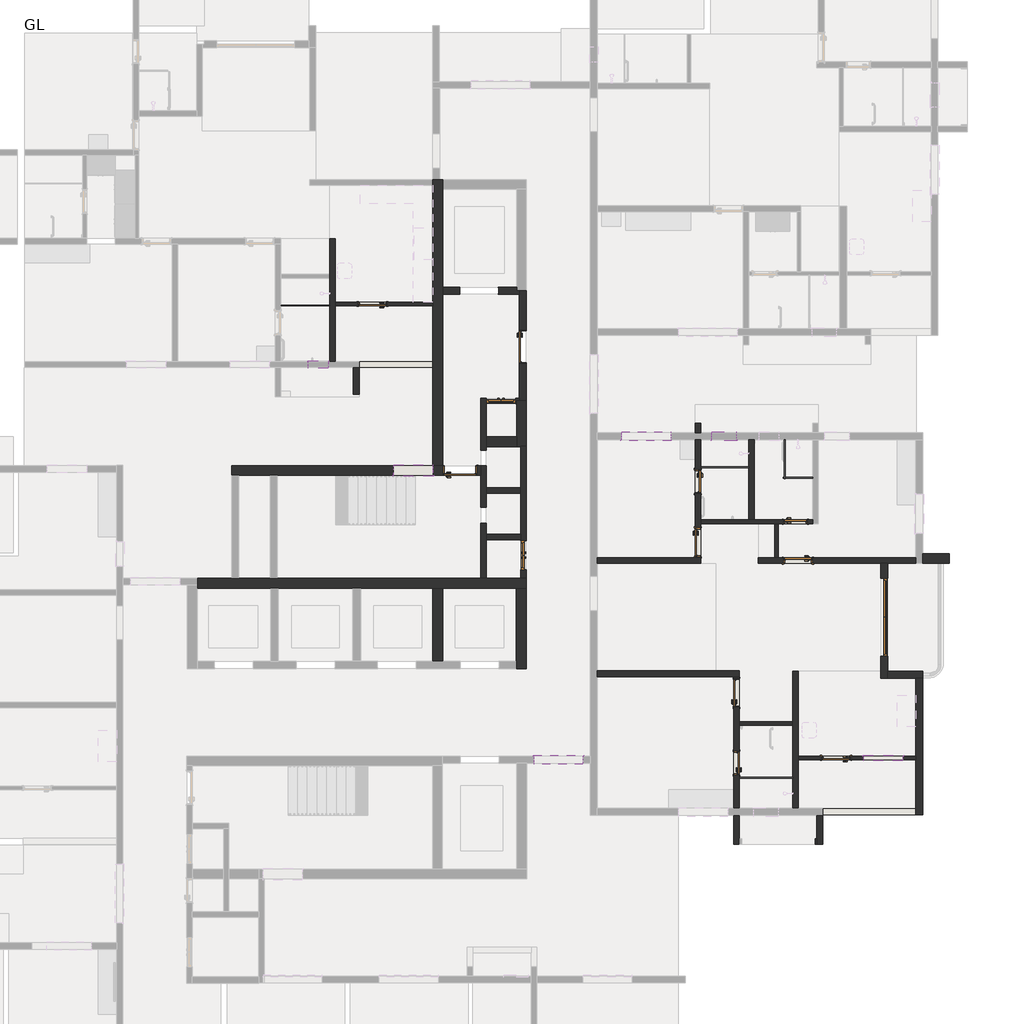
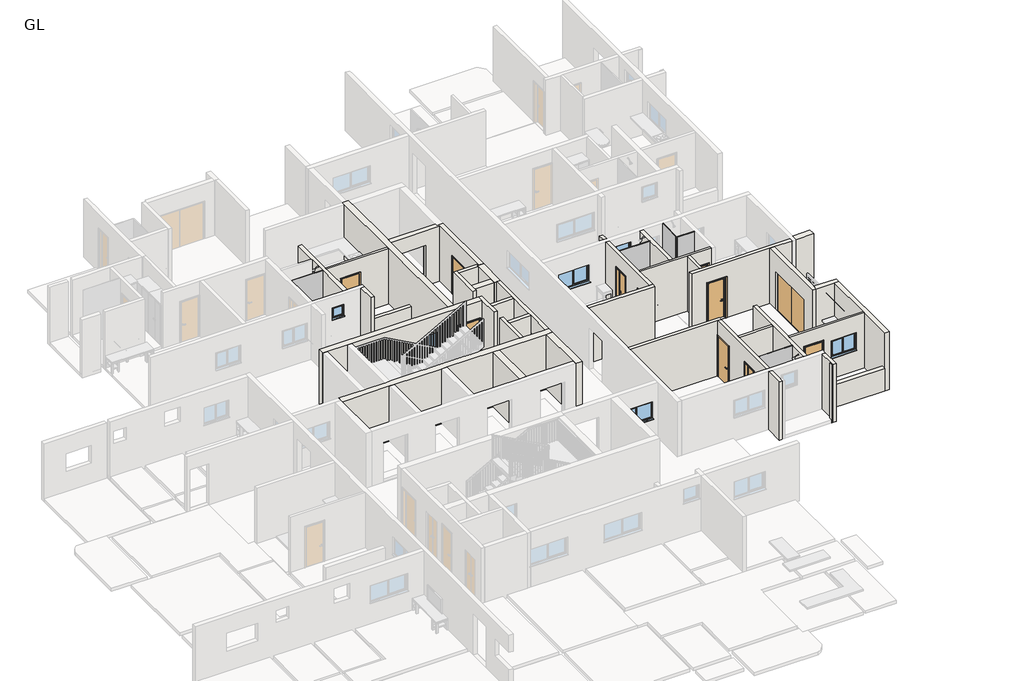
# One storey, part 5 of 14: 39 walls, 13 doors, 6 windows, 5 plates.
"""IFC4 building model written with IfcOpenShell, lengths in millimetres."""

from ifc_helpers import new_model, si_unit, frame, origin, origin_with_axes, place, context, project, spatial, polyline, outline, extrude, faceted_brep, transform, mapped, element, save
from components import doors_concept_extdbl_8_449e5563, doors_extdbl_flush_3_1e4ff7a8, doors_intsgl_2_5_door_21b53886, doors_intsgl_2_5_door_ce04bd24, doors_intsgl_2_5_door_fd097d29, doors_intsgl_3_door_8261d8fb, doors_intsgl_3_door_f61d7fb9, doors_intsgl_3_door_77e94e6e, doors_intsgl_3_5_f2e8c556, doors_intsgl_3_5_83ebdd9c, system_panel_glazed_f5bfe384, system_panel_glazed_a7f3818b, system_panel_glazed_4e5522aa, system_panel_glazed_8fd4c810, system_panel_glazed_557224e7, windows_dbl_plain_4_ad201dc9, windows_dbl_plain_4_4767a56f, windows_dbl_plain_5_907a13a5, windows_dbl_plain_5_93ba300c, windows_sgl_plain_2_43817c1b, windows_sgl_plain_2_5_21186da1

model = new_model("IFC4")

# Units and contexts
model_context = context("Model", 3, world=origin())
ifc_project = project(units=[si_unit("LENGTHUNIT", "METRE", prefix="MILLI")], contexts=[model_context])

# Site, building, storey
site = spatial("IfcSite", under=ifc_project)
building = spatial("IfcBuilding", under=site)
storey = spatial("IfcBuildingStorey", under=building, Name="GL", Elevation=0.0)

# Doors
placement = place(None, origin())
doors_concept_extdbl_8_shape = doors_concept_extdbl_8_449e5563(model_context)
element("IfcDoor", 1, ObjectType="Doors_Concept_ExtDbl : 8'", at=placement, inside=storey, context=model_context, shape_type="MappedRepresentation", body=[
    mapped(doors_concept_extdbl_8_shape, transform((18469.2769726, 77729.0878957, 0.0), x_axis=(0.0, -1.0, 0.0), y_axis=(1.0, 0.0, 0.0), z_axis=(0.0, 0.0, 1.0))),
])
doors_extdbl_flush_3_shape = doors_extdbl_flush_3_1e4ff7a8(model_context)
element("IfcDoor", 2, ObjectType="Doors_ExtDbl_Flush : 3'", at=placement, inside=storey, context=model_context, shape_type="MappedRepresentation", body=[
    mapped(doors_extdbl_flush_3_shape, transform((6505.8928654, 84487.5807724, 0.0), x_axis=(-1.0, 0.0, 0.0), y_axis=(0.0, -1.0, 0.0), z_axis=(0.0, 0.0, 1.0))),
])
element("IfcDoor", 3, ObjectType="Doors_ExtDbl_Flush : 3'", at=placement, inside=storey, context=model_context, shape_type="MappedRepresentation", body=[
    mapped(doors_extdbl_flush_3_shape, transform((7204.1388654, 79670.2853985, 0.0), x_axis=(0.0, 1.0, 0.0), y_axis=(-1.0, 0.0, 0.0), z_axis=(0.0, 0.0, 1.0))),
])
doors_intsgl_2_5_door_shape = doors_intsgl_2_5_door_21b53886(model_context)
element("IfcDoor", 4, ObjectType="Doors_IntSgl : 2.5' DOOR", at=placement, inside=storey, context=model_context, shape_type="MappedRepresentation", body=[
    mapped(doors_intsgl_2_5_door_shape, transform((15698.5624579, 80714.8578957, 149.9616), x_axis=(1.0, 0.0, 0.0), y_axis=(0.0, 1.0, 0.0), z_axis=(0.0, 0.0, 1.0))),
])
doors_intsgl_2_5_door_2_shape = doors_intsgl_2_5_door_ce04bd24(model_context)
element("IfcDoor", 5, ObjectType="Doors_IntSgl : 2.5' DOOR", at=placement, inside=storey, context=model_context, shape_type="MappedRepresentation", body=[
    mapped(doors_intsgl_2_5_door_2_shape, transform((12650.3084579, 81965.8078957, 149.9616), x_axis=(0.0, -1.0, 0.0), y_axis=(1.0, 0.0, 0.0), z_axis=(0.0, 0.0, 1.0))),
])
doors_intsgl_2_5_door_3_shape = doors_intsgl_2_5_door_fd097d29(model_context)
element("IfcDoor", 6, ObjectType="Doors_IntSgl : 2.5' DOOR", at=placement, inside=storey, context=model_context, shape_type="MappedRepresentation", body=[
    mapped(doors_intsgl_2_5_door_3_shape, transform((13856.9483556, 73179.9478957, 149.9616), x_axis=(0.0, 1.0, 0.0), y_axis=(-1.0, 0.0, 0.0), z_axis=(0.0, 0.0, 1.0))),
])
doors_intsgl_3_door_shape = doors_intsgl_3_door_8261d8fb(model_context)
element("IfcDoor", 7, ObjectType="Doors_IntSgl : 3' DOOR", at=placement, inside=storey, context=model_context, shape_type="MappedRepresentation", body=[
    mapped(doors_intsgl_3_door_shape, transform((12650.3084579, 80069.4438957, 149.9616), x_axis=(0.0, -1.0, 0.0), y_axis=(1.0, 0.0, 0.0), z_axis=(0.0, 0.0, 1.0))),
])
element("IfcDoor", 8, ObjectType="Doors_IntSgl : 3' DOOR", at=placement, inside=storey, context=model_context, shape_type="MappedRepresentation", body=[
    mapped(doors_intsgl_3_door_shape, transform((15774.7624579, 79499.9758957, 149.9616), x_axis=(-1.0, 0.0, 0.0), y_axis=(0.0, -1.0, 0.0), z_axis=(0.0, 0.0, 1.0))),
])
doors_intsgl_3_door_2_shape = doors_intsgl_3_door_f61d7fb9(model_context)
element("IfcDoor", 9, ObjectType="Doors_IntSgl : 3' DOOR", at=placement, inside=storey, context=model_context, shape_type="MappedRepresentation", body=[
    mapped(doors_intsgl_3_door_2_shape, transform((13856.9483556, 75373.5131416, 149.9616), x_axis=(0.0, 1.0, 0.0), y_axis=(-1.0, 0.0, 0.0), z_axis=(0.0, 0.0, 1.0))),
])
doors_intsgl_3_door_3_shape = doors_intsgl_3_door_77e94e6e(model_context)
element("IfcDoor", 10, ObjectType="Doors_IntSgl : 3' DOOR", at=placement, inside=storey, context=model_context, shape_type="MappedRepresentation", body=[
    mapped(doors_intsgl_3_door_3_shape, transform((16965.5969726, 73341.2378957, 149.9616), x_axis=(-1.0, 0.0, 0.0), y_axis=(0.0, -1.0, 0.0), z_axis=(0.0, 0.0, 1.0))),
])
element("IfcDoor", 11, ObjectType="Doors_IntSgl : 3' DOOR", at=placement, inside=storey, context=model_context, shape_type="MappedRepresentation", body=[
    mapped(doors_intsgl_3_door_3_shape, transform((2499.105001, 87511.7462935, 149.9616), x_axis=(-1.0, 0.0, 0.0), y_axis=(0.0, -1.0, 0.0), z_axis=(0.0, 0.0, 1.0))),
])
doors_intsgl_3_5_shape = doors_intsgl_3_5_f2e8c556(model_context)
element("IfcDoor", 12, ObjectType="Doors_IntSgl : 3.5'", at=placement, inside=storey, context=model_context, shape_type="MappedRepresentation", body=[
    mapped(doors_intsgl_3_5_shape, transform((5227.4968521, 82310.1073985, 0.0), x_axis=(1.0, 0.0, 0.0), y_axis=(0.0, 1.0, 0.0), z_axis=(0.0, 0.0, 1.0))),
])
doors_intsgl_3_5_2_shape = doors_intsgl_3_5_83ebdd9c(model_context)
element("IfcDoor", 13, ObjectType="Doors_IntSgl : 3.5'", at=placement, inside=storey, context=model_context, shape_type="MappedRepresentation", body=[
    mapped(doors_intsgl_3_5_2_shape, transform((7183.0568654, 86175.1982935, 0.0), x_axis=(0.0, -1.0, 0.0), y_axis=(1.0, 0.0, 0.0), z_axis=(0.0, 0.0, 1.0))),
])

# Plates
system_panel_glazed_shape = system_panel_glazed_f5bfe384(model_context)
element("IfcPlate", 14, ObjectType="System Panel : Glazed", at=placement, inside=storey, context=model_context, shape_type="MappedRepresentation", body=[
    mapped(system_panel_glazed_shape, transform((14789.4512792, 72687.7478957, 0.0), x_axis=(1.0, 0.0, 0.0), y_axis=(0.0, 1.0, 0.0), z_axis=(0.0, 0.0, 1.0))),
])
system_panel_glazed_2_shape = system_panel_glazed_a7f3818b(model_context)
element("IfcPlate", 15, ObjectType="System Panel : Glazed", at=placement, inside=storey, context=model_context, shape_type="MappedRepresentation", body=[
    mapped(system_panel_glazed_2_shape, transform((13499.6514579, 82381.8078957, 0.0), x_axis=(1.0, 0.0, 0.0), y_axis=(0.0, 1.0, 0.0), z_axis=(0.0, 0.0, 1.0))),
])
system_panel_glazed_3_shape = system_panel_glazed_4e5522aa(model_context)
element("IfcPlate", 16, ObjectType="System Panel : Glazed", at=placement, inside=storey, context=model_context, shape_type="MappedRepresentation", body=[
    mapped(system_panel_glazed_3_shape, transform((15323.9124579, 82664.3078957, 0.0), x_axis=(0.0, -1.0, 0.0), y_axis=(1.0, 0.0, 0.0), z_axis=(0.0, 0.0, 1.0))),
])
system_panel_glazed_4_shape = system_panel_glazed_8fd4c810(model_context)
element("IfcPlate", 17, ObjectType="System Panel : Glazed", at=placement, inside=storey, context=model_context, shape_type="MappedRepresentation", body=[
    mapped(system_panel_glazed_4_shape, transform((15777.9374579, 82054.7078957, 0.0), x_axis=(1.0, 0.0, 0.0), y_axis=(0.0, 1.0, 0.0), z_axis=(0.0, 0.0, 1.0))),
])
system_panel_glazed_5_shape = system_panel_glazed_557224e7(model_context)
element("IfcPlate", 18, ObjectType="System Panel : Glazed", at=placement, inside=storey, context=model_context, shape_type="MappedRepresentation", body=[
    mapped(system_panel_glazed_5_shape, transform((392.537001, 87429.1962935, 0.0), x_axis=(1.0, 0.0, 0.0), y_axis=(0.0, 1.0, 0.0), z_axis=(0.0, 0.0, 1.0))),
])

# Walls
element("IfcWall", 19, ObjectType="W2", at=placement, inside=storey, context=model_context, shape_type="Brep", body=[
    faceted_brep([(19454.7969726, 79586.8438957, 0.0), (15165.1624579, 79586.8438957, 0.0), (15050.8624579, 79586.8438957, 0.0), (14537.3569726, 79586.8438957, 0.0), (14537.3569726, 79586.8438957, 3000.0), (15050.8624579, 79586.8438957, 3000.0), (15165.1624579, 79586.8438957, 3000.0), (19454.7969726, 79586.8438957, 3000.0), (15317.5624579, 79586.8438957, 2259.9616), (15317.5624579, 79586.8438957, 149.9616), (16231.9624579, 79586.8438957, 149.9616), (16231.9624579, 79586.8438957, 2259.9616), (14537.3569726, 79413.1078957, 0.0), (18362.5969726, 79413.1078957, 0.0), (18575.9569726, 79413.1078957, 0.0), (19454.7969726, 79413.1078957, 0.0), (19454.7969726, 79413.1078957, 3000.0), (18575.9569726, 79413.1078957, 3000.0), (18362.5969726, 79413.1078957, 3000.0), (14537.3569726, 79413.1078957, 3000.0), (15317.5624579, 79413.1078957, 149.9616), (15317.5624579, 79413.1078957, 2259.9616), (16231.9624579, 79413.1078957, 2259.9616), (16231.9624579, 79413.1078957, 149.9616)], [[[0, 1, 2, 3, 4, 5, 6, 7], [8, 9, 10, 11]], [[12, 13, 14, 15, 16, 17, 18, 19], [20, 21, 22, 23]], [[3, 2, 1, 0, 15, 14, 13, 12]], [[4, 3, 12, 19]], [[7, 6, 5, 4, 19, 18, 17, 16]], [[0, 7, 16, 15]], [[20, 9, 8, 21]], [[21, 8, 11, 22]], [[22, 11, 10, 23]], [[9, 20, 23, 10]]]),
])
element("IfcWall", 20, ObjectType="W2", at=placement, inside=storey, context=model_context, shape_type="Brep", body=[
    faceted_brep([(12737.1764579, 79586.8438957, 0.0), (12563.4404579, 79586.8438957, 0.0), (9508.1569726, 79586.8438957, 0.0), (9508.1569726, 79586.8438957, 3000.0), (12563.4404579, 79586.8438957, 3000.0), (12737.1764579, 79586.8438957, 3000.0), (12737.1764579, 79413.1078957, 0.0), (12737.1764579, 79413.1078957, 3000.0), (9508.1569726, 79413.1078957, 3000.0), (9508.1569726, 79413.1078957, 0.0)], [[[0, 1, 2, 3, 4, 5]], [[6, 7, 8, 9]], [[2, 1, 0, 6, 9]], [[5, 4, 3, 8, 7]], [[3, 2, 9, 8]], [[0, 5, 7, 6]]]),
])
element("IfcWall", 21, ObjectType="W2", at=placement, inside=storey, context=model_context, shape_type="Brep", body=[
    faceted_brep([(15615.0862029, 76050.1478957, 0.0), (15615.0862029, 74475.3478957, 0.0), (15615.0862029, 74361.0478957, 0.0), (15615.0862029, 71762.6278957, 0.0), (15615.0862029, 71762.6278957, 3000.0), (15615.0862029, 74361.0478957, 3000.0), (15615.0862029, 74475.3478957, 3000.0), (15615.0862029, 76050.1478957, 3000.0), (15788.8222029, 76050.1478957, 0.0), (15788.8222029, 76050.1478957, 3000.0), (15788.8222029, 73398.3878957, 3000.0), (15788.8222029, 73284.0878957, 3000.0), (15788.8222029, 71762.6278957, 3000.0), (15788.8222029, 71762.6278957, 0.0), (15788.8222029, 73284.0878957, 0.0), (15788.8222029, 73398.3878957, 0.0)], [[[0, 1, 2, 3, 4, 5, 6, 7]], [[8, 9, 10, 11, 12, 13, 14, 15]], [[3, 2, 1, 0, 8, 15, 14, 13]], [[7, 6, 5, 4, 12, 11, 10, 9]], [[0, 7, 9, 8]], [[4, 3, 13, 12]]]),
])
element("IfcWall", 22, ObjectType="W2", at=placement, inside=storey, context=model_context, shape_type="Brep", body=[
    faceted_brep([(13943.8163556, 76055.2491416, 0.0), (9508.1569726, 76055.2491416, 0.0), (9508.1569726, 76055.2491416, 3000.0), (13943.8163556, 76055.2491416, 3000.0), (13943.8163556, 75881.5131416, 0.0), (13943.8163556, 75881.5131416, 3000.0), (13770.0803556, 75881.5131416, 3000.0), (9508.1569726, 75881.5131416, 3000.0), (9508.1569726, 75881.5131416, 0.0), (13770.0803556, 75881.5131416, 0.0)], [[[0, 1, 2, 3]], [[4, 5, 6, 7, 8, 9]], [[1, 0, 4, 9, 8]], [[3, 2, 7, 6, 5]], [[2, 1, 8, 7]], [[0, 3, 5, 4]]]),
])
element("IfcWall", 23, ObjectType="W2", at=placement, inside=storey, context=model_context, shape_type="Brep", body=[
    faceted_brep([(13770.0803556, 75881.5131416, 3000.0), (13770.0803556, 75881.5131416, 0.0), (13770.0803556, 71762.6278957, 0.0), (13770.0803556, 71762.6278957, 3000.0), (13770.0803556, 75830.7131416, 149.9616), (13770.0803556, 75830.7131416, 2259.9616), (13770.0803556, 74916.3131416, 2259.9616), (13770.0803556, 74916.3131416, 149.9616), (13770.0803556, 73560.9478957, 149.9616), (13770.0803556, 73560.9478957, 2259.9616), (13770.0803556, 72798.9478957, 2259.9616), (13770.0803556, 72798.9478957, 149.9616), (13943.8163556, 75881.5131416, 0.0), (13943.8163556, 75881.5131416, 3000.0), (13943.8163556, 74475.3478957, 3000.0), (13943.8163556, 74361.0478957, 3000.0), (13943.8163556, 71762.6278957, 3000.0), (13943.8163556, 71762.6278957, 0.0), (13943.8163556, 74361.0478957, 0.0), (13943.8163556, 74475.3478957, 0.0), (13943.8163556, 75830.7131416, 2259.9616), (13943.8163556, 75830.7131416, 149.9616), (13943.8163556, 74916.3131416, 149.9616), (13943.8163556, 74916.3131416, 2259.9616), (13943.8163556, 73560.9478957, 2259.9616), (13943.8163556, 73560.9478957, 149.9616), (13943.8163556, 72798.9478957, 149.9616), (13943.8163556, 72798.9478957, 2259.9616)], [[[0, 1, 2, 3], [4, 5, 6, 7], [8, 9, 10, 11]], [[12, 13, 14, 15, 16, 17, 18, 19], [20, 21, 22, 23], [24, 25, 26, 27]], [[1, 12, 19, 18, 17, 2]], [[13, 0, 3, 16, 15, 14]], [[1, 0, 13, 12]], [[3, 2, 17, 16]], [[4, 21, 20, 5]], [[5, 20, 23, 6]], [[22, 7, 6, 23]], [[21, 4, 7, 22]], [[8, 25, 24, 9]], [[9, 24, 27, 10]], [[26, 11, 10, 27]], [[25, 8, 11, 26]]]),
    faceted_brep([(13770.0803556, 70638.9318957, 0.0), (13770.0803556, 70638.9318957, 3000.0), (13770.0803556, 71549.2678957, 3000.0), (13770.0803556, 71549.2678957, 0.0), (13943.8163556, 70638.9318957, 3000.0), (13943.8163556, 70638.9318957, 0.0), (13943.8163556, 70812.6678957, 0.0), (13943.8163556, 71549.2678957, 0.0), (13943.8163556, 71549.2678957, 3000.0), (13943.8163556, 70812.6678957, 3000.0)], [[[0, 1, 2, 3]], [[4, 5, 6, 7, 8, 9]], [[5, 0, 3, 7, 6]], [[1, 4, 9, 8, 2]], [[3, 2, 8, 7]], [[1, 0, 5, 4]]]),
])
element("IfcWall", 24, ObjectType="W2", at=placement, inside=storey, context=model_context, shape_type="Brep", body=[
    faceted_brep([(16370.2209726, 71549.2678957, 0.0), (16370.2209726, 70812.6678957, 0.0), (16370.2209726, 70638.9318957, 0.0), (16370.2209726, 70638.9318957, 3000.0), (16370.2209726, 70812.6678957, 3000.0), (16370.2209726, 71549.2678957, 3000.0), (16543.9569726, 71549.2678957, 0.0), (16543.9569726, 71549.2678957, 3000.0), (16543.9569726, 70638.9318957, 3000.0), (16543.9569726, 70638.9318957, 0.0)], [[[0, 1, 2, 3, 4, 5]], [[6, 7, 8, 9]], [[2, 1, 0, 6, 9]], [[5, 4, 3, 8, 7]], [[0, 5, 7, 6]], [[3, 2, 9, 8]]]),
])
element("IfcWall", 25, ObjectType="W2", at=placement, inside=storey, context=model_context, shape_type="SweptSolid", body=[
    extrude(outline(polyline([(14242.1264579, 80772.0078957), (14242.1264579, 83273.9078957), (14415.8624579, 83273.9078957), (14415.8624579, 80772.0078957), (14242.1264579, 80772.0078957)])), origin_with_axes(), (0.0, 0.0, 1.0), 3000.0),
])
element("IfcWall", 26, ObjectType="W2", at=placement, inside=storey, context=model_context, shape_type="Brep", body=[
    faceted_brep([(12563.4404579, 83273.9078957, 0.0), (12563.4404579, 79586.8438957, 0.0), (12563.4404579, 79586.8438957, 3000.0), (12563.4404579, 83273.9078957, 3000.0), (12563.4404579, 79612.2438957, 2259.9616), (12563.4404579, 79612.2438957, 149.9616), (12563.4404579, 80526.6438957, 149.9616), (12563.4404579, 80526.6438957, 2259.9616), (12563.4404579, 81584.8078957, 2259.9616), (12563.4404579, 81584.8078957, 149.9616), (12563.4404579, 82346.8078957, 149.9616), (12563.4404579, 82346.8078957, 2259.9616), (12737.1764579, 79586.8438957, 0.0), (12737.1764579, 80657.7078957, 0.0), (12737.1764579, 80772.0078957, 0.0), (12737.1764579, 83273.9078957, 0.0), (12737.1764579, 83273.9078957, 3000.0), (12737.1764579, 80772.0078957, 3000.0), (12737.1764579, 80657.7078957, 3000.0), (12737.1764579, 79586.8438957, 3000.0), (12737.1764579, 79612.2438957, 149.9616), (12737.1764579, 79612.2438957, 2259.9616), (12737.1764579, 80526.6438957, 2259.9616), (12737.1764579, 80526.6438957, 149.9616), (12737.1764579, 81584.8078957, 149.9616), (12737.1764579, 81584.8078957, 2259.9616), (12737.1764579, 82346.8078957, 2259.9616), (12737.1764579, 82346.8078957, 149.9616)], [[[0, 1, 2, 3], [4, 5, 6, 7], [8, 9, 10, 11]], [[12, 13, 14, 15, 16, 17, 18, 19], [20, 21, 22, 23], [24, 25, 26, 27]], [[1, 0, 15, 14, 13, 12]], [[3, 2, 19, 18, 17, 16]], [[2, 1, 12, 19]], [[0, 3, 16, 15]], [[20, 5, 4, 21]], [[21, 4, 7, 22]], [[22, 7, 6, 23]], [[5, 20, 23, 6]], [[24, 9, 8, 25]], [[25, 8, 11, 26]], [[10, 27, 26, 11]], [[9, 24, 27, 10]]]),
])
element("IfcWall", 27, ObjectType="W2", at=placement, inside=storey, context=model_context, shape_type="SweptSolid", body=[
    extrude(outline(polyline([(16319.4209726, 70812.6678957), (16370.2209726, 70812.6678957), (16370.2209726, 70638.9318957), (16319.4209726, 70638.9318957), (16319.4209726, 70812.6678957)])), origin_with_axes(), (0.0, 0.0, 1.0), 3000.0),
])
element("IfcWall", 28, ObjectType="W2", at=placement, inside=storey, context=model_context, shape_type="SweptSolid", body=[
    extrude(outline(polyline([(4366.005001, 85538.1556254), (2080.005001, 85538.1556254), (2080.005001, 85711.8916254), (4366.005001, 85711.8916254), (4366.005001, 85538.1556254)])), origin_with_axes(), (0.0, 0.0, 1.0), 1171.2),
])
element("IfcWall", 29, ObjectType="W2", at=placement, inside=storey, context=model_context, shape_type="Brep", body=[
    faceted_brep([(7291.0068654, 80127.4853985, 2110.0), (7291.0068654, 80127.4853985, 0.0), (7291.0068654, 83063.1487724, 0.0), (7291.0068654, 83063.1487724, 3000.0), (7291.0068654, 78948.3487724, 3000.0), (7291.0068654, 78948.3487724, 0.0), (7291.0068654, 79213.0853985, 0.0), (7291.0068654, 79213.0853985, 2110.0), (7117.2708654, 83063.1487724, 0.0), (7117.2708654, 81776.7073985, 0.0), (7117.2708654, 81602.9713985, 0.0), (7117.2708654, 80326.6213985, 0.0), (7117.2708654, 80152.8853985, 0.0), (7117.2708654, 80127.4853985, 0.0), (7117.2708654, 80127.4853985, 2110.0), (7117.2708654, 79213.0853985, 2110.0), (7117.2708654, 79213.0853985, 0.0), (7117.2708654, 78948.3487724, 0.0), (7117.2708654, 78948.3487724, 3000.0), (7117.2708654, 80152.8853985, 3000.0), (7117.2708654, 80326.6213985, 3000.0), (7117.2708654, 81602.9713985, 3000.0), (7117.2708654, 81776.7073985, 3000.0), (7117.2708654, 83063.1487724, 3000.0)], [[[0, 1, 2, 3, 4, 5, 6, 7]], [[8, 9, 10, 11, 12, 13, 14, 15, 16, 17, 18, 19, 20, 21, 22, 23]], [[6, 5, 17, 16]], [[2, 1, 13, 12, 11, 10, 9, 8]], [[3, 2, 8, 23]], [[4, 3, 23, 22, 21, 20, 19, 18]], [[5, 4, 18, 17]], [[16, 15, 7, 6]], [[14, 13, 1, 0]], [[15, 14, 0, 7]]]),
])
element("IfcWall", 30, ObjectType="W2", at=placement, inside=storey, context=model_context, shape_type="Brep", body=[
    faceted_brep([(6048.6928654, 78948.3487724, 0.0), (6048.6928654, 80152.8853985, 0.0), (6048.6928654, 80326.6213985, 0.0), (6048.6928654, 80662.8487724, 0.0), (6048.6928654, 80662.8487724, 3000.0), (6048.6928654, 80326.6213985, 3000.0), (6048.6928654, 80152.8853985, 3000.0), (6048.6928654, 78948.3487724, 3000.0), (5874.9568654, 78948.3487724, 0.0), (5874.9568654, 78948.3487724, 3000.0), (5874.9568654, 80662.8487724, 3000.0), (5874.9568654, 80662.8487724, 0.0)], [[[0, 1, 2, 3, 4, 5, 6, 7]], [[8, 9, 10, 11]], [[3, 2, 1, 0, 8, 11]], [[4, 3, 11, 10]], [[7, 6, 5, 4, 10, 9]], [[0, 7, 9, 8]]]),
])
element("IfcWall", 31, ObjectType="W2", at=placement, inside=storey, context=model_context, shape_type="Brep", body=[
    faceted_brep([(6992.5568654, 84400.7127724, 3000.0), (6048.6928654, 84400.7127724, 3000.0), (6048.6928654, 84400.7127724, 2110.0), (6963.0928654, 84400.7127724, 2110.0), (6963.0928654, 84400.7127724, 0.0), (6992.5568654, 84400.7127724, 0.0), (7068.7568654, 84574.4487724, 3000.0), (7068.7568654, 84574.4487724, 0.0), (6963.0928654, 84574.4487724, 0.0), (6963.0928654, 84574.4487724, 2110.0), (6048.6928654, 84574.4487724, 2110.0), (6048.6928654, 84574.4487724, 3000.0), (7068.7568654, 84487.5807724, 0.0), (6992.5568654, 84487.5807724, 0.0), (6992.5568654, 84487.5807724, 3000.0), (7068.7568654, 84487.5807724, 3000.0)], [[[0, 1, 2, 3, 4, 5]], [[6, 7, 8, 9, 10, 11]], [[7, 12, 13, 5, 4, 8]], [[1, 0, 14, 15, 6, 11]], [[0, 5, 13, 14]], [[13, 12, 15, 14]], [[7, 6, 15, 12]], [[1, 11, 10, 2]], [[3, 9, 8, 4]], [[9, 3, 2, 10]]]),
])
element("IfcWall", 32, ObjectType="W2", at=placement, inside=storey, context=model_context, shape_type="Brep", body=[
    faceted_brep([(1330.705001, 85711.8916254, 0.0), (1330.705001, 87454.5962935, 0.0), (1330.705001, 87568.8962935, 0.0), (1330.705001, 89553.6416254, 0.0), (1330.705001, 89553.6416254, 3000.0), (1330.705001, 87568.8962935, 3000.0), (1330.705001, 87454.5962935, 3000.0), (1330.705001, 85711.8916254, 3000.0), (1156.969001, 85711.8916254, 0.0), (1156.969001, 85711.8916254, 3000.0), (1156.969001, 88321.7416254, 3000.0), (1156.969001, 88436.0416254, 3000.0), (1156.969001, 89553.6416254, 3000.0), (1156.969001, 89553.6416254, 0.0), (1156.969001, 88436.0416254, 0.0), (1156.969001, 88321.7416254, 0.0)], [[[0, 1, 2, 3, 4, 5, 6, 7]], [[8, 9, 10, 11, 12, 13, 14, 15]], [[3, 2, 1, 0, 8, 15, 14, 13]], [[4, 3, 13, 12]], [[7, 6, 5, 4, 12, 11, 10, 9]], [[0, 7, 9, 8]]]),
])
element("IfcWall", 33, ObjectType="W2", at=placement, inside=storey, context=model_context, shape_type="SweptSolid", body=[
    extrude(outline(polyline([(1899.919001, 84697.9236254), (1899.919001, 85538.1556254), (2073.655001, 85538.1556254), (2073.655001, 84697.9236254), (1899.919001, 84697.9236254)])), origin_with_axes(), (0.0, 0.0, 1.0), 3000.0),
])
element("IfcWall", 34, ObjectType="W2", at=placement, inside=storey, context=model_context, shape_type="Brep", body=[
    faceted_brep([(6048.6928654, 82948.8487724, 0.0), (6048.6928654, 83056.7987724, 0.0), (6048.6928654, 83361.5987724, 0.0), (6048.6928654, 84574.4487724, 0.0), (6048.6928654, 84574.4487724, 2110.0), (6048.6928654, 84574.4487724, 3000.0), (6048.6928654, 84400.7127724, 3000.0), (6048.6928654, 83361.5987724, 3000.0), (6048.6928654, 83056.7987724, 3000.0), (6048.6928654, 82948.8487724, 3000.0), (5874.9568654, 82948.8487724, 0.0), (5874.9568654, 82948.8487724, 3000.0), (5874.9568654, 84574.4487724, 3000.0), (5874.9568654, 84574.4487724, 0.0)], [[[0, 1, 2, 3, 4, 5, 6, 7, 8, 9]], [[10, 11, 12, 13]], [[3, 2, 1, 0, 10, 13]], [[9, 8, 7, 6, 5, 12, 11]], [[0, 9, 11, 10]], [[5, 4, 3, 13, 12]]]),
])
element("IfcWall", 35, ObjectType="W2", at=placement, inside=storey, context=model_context, shape_type="Brep", body=[
    faceted_brep([(6048.6928654, 81170.8487724, 0.0), (6048.6928654, 81602.9713985, 0.0), (6048.6928654, 81776.7073985, 0.0), (6048.6928654, 82466.2487724, 0.0), (6048.6928654, 82466.2487724, 3000.0), (6048.6928654, 81776.7073985, 3000.0), (6048.6928654, 81602.9713985, 3000.0), (6048.6928654, 81170.8487724, 3000.0), (5874.9568654, 81170.8487724, 0.0), (5874.9568654, 81170.8487724, 3000.0), (5874.9568654, 82157.7073985, 3000.0), (5874.9568654, 82462.5073985, 3000.0), (5874.9568654, 82466.2487724, 3000.0), (5874.9568654, 82466.2487724, 0.0), (5874.9568654, 82462.5073985, 0.0), (5874.9568654, 82157.7073985, 0.0)], [[[0, 1, 2, 3, 4, 5, 6, 7]], [[8, 9, 10, 11, 12, 13, 14, 15]], [[3, 2, 1, 0, 8, 15, 14, 13]], [[4, 3, 13, 12]], [[7, 6, 5, 4, 12, 11, 10, 9]], [[0, 7, 9, 8]]]),
])
element("IfcWall", 36, ObjectType="W2", at=placement, inside=storey, context=model_context, shape_type="SweptSolid", body=[
    extrude(outline(polyline([(6048.6928654, 81776.7073985), (7117.2708654, 81776.7073985), (7117.2708654, 81602.9713985), (6048.6928654, 81602.9713985), (6048.6928654, 81776.7073985)])), origin_with_axes(), (0.0, 0.0, 1.0), 3000.0),
])
element("IfcWall", 37, ObjectType="W2", at=placement, inside=storey, context=model_context, shape_type="SweptSolid", body=[
    extrude(outline(polyline([(6048.6928654, 80326.6213985), (7117.2708654, 80326.6213985), (7117.2708654, 80152.8853985), (6048.6928654, 80152.8853985), (6048.6928654, 80326.6213985)])), origin_with_axes(), (0.0, 0.0, 1.0), 3000.0),
])
element("IfcWall", 38, ObjectType="W2", at=placement, inside=storey, context=model_context, shape_type="SweptSolid", body=[
    extrude(outline(polyline([(12737.1764579, 83792.0678957), (12737.1764579, 83487.2678957), (12563.4404579, 83487.2678957), (12563.4404579, 83792.0678957), (12737.1764579, 83792.0678957)])), origin_with_axes(), (0.0, 0.0, 1.0), 3000.0),
])
element("IfcWall", 39, ObjectType="W3", at=placement, inside=storey, context=model_context, shape_type="SweptSolid", body=[
    extrude(outline(polyline([(0.0, 15788.8222029), (0.0, 19454.7969726), (3000.0, 19454.7969726), (3000.0, 15788.8222029), (0.0, 15788.8222029)]), holes=[polyline([(2110.0, 19048.3969726), (1200.0, 19048.3969726), (1200.0, 17829.1969726), (2110.0, 17829.1969726), (2110.0, 19048.3969726)]), polyline([(149.9616, 16508.3969726), (2259.9616, 16508.3969726), (2259.9616, 17422.7969726), (149.9616, 17422.7969726), (149.9616, 16508.3969726)])]), frame((0.0, 73284.0878957, 0.0), z_axis=(0.0, 1.0, 0.0), x_axis=(0.0, 0.0, 1.0)), (0.0, 0.0, 1.0), 114.3),
])
element("IfcWall", 40, ObjectType="W3", at=placement, inside=storey, context=model_context, shape_type="Brep", body=[
    faceted_brep([(16231.9624579, 80772.0078957, 0.0), (14415.8624579, 80772.0078957, 0.0), (14242.1264579, 80772.0078957, 0.0), (12737.1764579, 80772.0078957, 0.0), (12737.1764579, 80772.0078957, 3000.0), (14242.1264579, 80772.0078957, 3000.0), (14415.8624579, 80772.0078957, 3000.0), (16231.9624579, 80772.0078957, 3000.0), (16079.5624579, 80772.0078957, 149.9616), (16079.5624579, 80772.0078957, 2259.9616), (15317.5624579, 80772.0078957, 2259.9616), (15317.5624579, 80772.0078957, 149.9616), (12737.1764579, 80657.7078957, 0.0), (15050.8624579, 80657.7078957, 0.0), (15165.1624579, 80657.7078957, 0.0), (16231.9624579, 80657.7078957, 0.0), (16231.9624579, 80657.7078957, 3000.0), (15165.1624579, 80657.7078957, 3000.0), (15050.8624579, 80657.7078957, 3000.0), (12737.1764579, 80657.7078957, 3000.0), (16079.5624579, 80657.7078957, 2259.9616), (16079.5624579, 80657.7078957, 149.9616), (15317.5624579, 80657.7078957, 149.9616), (15317.5624579, 80657.7078957, 2259.9616)], [[[0, 1, 2, 3, 4, 5, 6, 7], [8, 9, 10, 11]], [[12, 13, 14, 15, 16, 17, 18, 19], [20, 21, 22, 23]], [[3, 2, 1, 0, 15, 14, 13, 12]], [[7, 6, 5, 4, 19, 18, 17, 16]], [[0, 7, 16, 15]], [[4, 3, 12, 19]], [[8, 21, 20, 9]], [[9, 20, 23, 10]], [[10, 23, 22, 11]], [[21, 8, 11, 22]]]),
])
element("IfcWall", 41, ObjectType="W3", at=placement, inside=storey, context=model_context, shape_type="SweptSolid", body=[
    extrude(outline(polyline([(13943.8163556, 74475.3478957), (15615.0862029, 74475.3478957), (15615.0862029, 74361.0478957), (13943.8163556, 74361.0478957), (13943.8163556, 74475.3478957)])), origin_with_axes(), (0.0, 0.0, 1.0), 3000.0),
])
element("IfcWall", 42, ObjectType="W3", at=placement, inside=storey, context=model_context, shape_type="SweptSolid", body=[
    extrude(outline(polyline([(15050.8624579, 79586.8438957), (15050.8624579, 80657.7078957), (15165.1624579, 80657.7078957), (15165.1624579, 79586.8438957), (15050.8624579, 79586.8438957)])), origin_with_axes(), (0.0, 0.0, 1.0), 3000.0),
])
element("IfcWall", 43, ObjectType="W3", at=placement, inside=storey, context=model_context, shape_type="SweptSolid", body=[
    extrude(outline(polyline([(0.0, 1330.705001), (0.0, 4376.8368387), (3000.0, 4376.8368387), (3000.0, 1330.705001), (0.0, 1330.705001)]), holes=[polyline([(149.9616, 2041.905001), (2259.9616, 2041.905001), (2259.9616, 2956.305001), (149.9616, 2956.305001), (149.9616, 2041.905001)])]), frame((0.0, 87454.5962935, 0.0), z_axis=(0.0, 1.0, 0.0), x_axis=(0.0, 0.0, 1.0)), (0.0, 0.0, 1.0), 114.3),
])
element("IfcWall", 44, ObjectType="W4", at=placement, inside=storey, context=model_context, shape_type="Brep", body=[
    faceted_brep([(-2983.2931346, 78643.5487724, 0.0), (-686.4678446, 78643.5487724, 0.0), (-442.6278446, 78643.5487724, 0.0), (1881.4721554, 78643.5487724, 0.0), (2125.3121554, 78643.5487724, 0.0), (4382.7068654, 78643.5487724, 0.0), (4687.5068654, 78643.5487724, 0.0), (6986.2068654, 78643.5487724, 0.0), (7291.0068654, 78643.5487724, 0.0), (7291.0068654, 78643.5487724, 3000.0), (6986.2068654, 78643.5487724, 3000.0), (4687.5068654, 78643.5487724, 3000.0), (4382.7068654, 78643.5487724, 3000.0), (2125.3121554, 78643.5487724, 3000.0), (1881.4721554, 78643.5487724, 3000.0), (-442.6278446, 78643.5487724, 3000.0), (-686.4678446, 78643.5487724, 3000.0), (-2983.2931346, 78643.5487724, 3000.0), (-2983.2931346, 78948.3487724, 0.0), (-2983.2931346, 78948.3487724, 3000.0), (-1903.3131613, 78948.3487724, 3000.0), (-1680.8091613, 78948.3487724, 3000.0), (-701.1311613, 78948.3487724, 3000.0), (-478.6271613, 78948.3487724, 3000.0), (5874.9568654, 78948.3487724, 3000.0), (6048.6928654, 78948.3487724, 3000.0), (7117.2708654, 78948.3487724, 3000.0), (7291.0068654, 78948.3487724, 3000.0), (7291.0068654, 78948.3487724, 0.0), (7117.2708654, 78948.3487724, 0.0), (6048.6928654, 78948.3487724, 0.0), (5874.9568654, 78948.3487724, 0.0), (-478.6271613, 78948.3487724, 0.0), (-701.1311613, 78948.3487724, 0.0), (-1680.8091613, 78948.3487724, 0.0), (-1903.3131613, 78948.3487724, 0.0), (-2983.2931346, 78750.2287724, 0.0), (-2983.2931346, 78750.2287724, 3000.0)], [[[0, 1, 2, 3, 4, 5, 6, 7, 8, 9, 10, 11, 12, 13, 14, 15, 16, 17]], [[18, 19, 20, 21, 22, 23, 24, 25, 26, 27, 28, 29, 30, 31, 32, 33, 34, 35]], [[8, 7, 6, 5, 4, 3, 2, 1, 0, 36, 18, 35, 34, 33, 32, 31, 30, 29, 28]], [[17, 16, 15, 14, 13, 12, 11, 10, 9, 27, 26, 25, 24, 23, 22, 21, 20, 19, 37]], [[0, 17, 37, 19, 18, 36]], [[9, 8, 28, 27]]]),
])
element("IfcWall", 45, ObjectType="W4", at=placement, inside=storey, context=model_context, shape_type="Brep", body=[
    faceted_brep([(6986.2068654, 78643.5487724, 0.0), (6986.2068654, 76353.9927724, 0.0), (6986.2068654, 76131.4887724, 0.0), (6986.2068654, 76131.4887724, 3000.0), (6986.2068654, 76353.9927724, 3000.0), (6986.2068654, 78643.5487724, 3000.0), (7291.0068654, 78643.5487724, 0.0), (7291.0068654, 78643.5487724, 3000.0), (7291.0068654, 76131.4887724, 3000.0), (7291.0068654, 76131.4887724, 0.0)], [[[0, 1, 2, 3, 4, 5]], [[6, 7, 8, 9]], [[2, 1, 0, 6, 9]], [[5, 4, 3, 8, 7]], [[0, 5, 7, 6]], [[3, 2, 9, 8]]]),
])
element("IfcWall", 46, ObjectType="W4", at=placement, inside=storey, context=model_context, shape_type="SweptSolid", body=[
    extrude(outline(polyline([(4382.7068654, 76353.9927724), (4382.7068654, 78643.5487724), (4687.5068654, 78643.5487724), (4687.5068654, 76353.9927724), (4382.7068654, 76353.9927724)])), origin_with_axes(), (0.0, 0.0, 1.0), 3000.0),
])
element("IfcWall", 47, ObjectType="W4", at=placement, inside=storey, context=model_context, shape_type="SweptSolid", body=[
    extrude(outline(polyline([(19668.1569726, 79717.9078957), (20506.3569726, 79717.9078957), (20506.3569726, 79413.1078957), (19668.1569726, 79413.1078957), (19668.1569726, 79717.9078957)])), origin_with_axes(), (0.0, 0.0, 1.0), 3000.0),
])
element("IfcWall", 48, ObjectType="W4", at=placement, inside=storey, context=model_context, shape_type="Brep", body=[
    faceted_brep([(4376.8368387, 91396.9573985, 0.0), (4376.8368387, 91223.2213985, 0.0), (4376.8368387, 87568.8962935, 0.0), (4376.8368387, 87454.5962935, 0.0), (4376.8368387, 82462.5073985, 0.0), (4376.8368387, 82462.5073985, 3000.0), (4376.8368387, 87454.5962935, 3000.0), (4376.8368387, 87568.8962935, 3000.0), (4376.8368387, 91223.2213985, 3000.0), (4376.8368387, 91396.9573985, 3000.0), (4681.6368387, 91396.9573985, 0.0), (4681.6368387, 91396.9573985, 3000.0), (4681.6368387, 91092.1573985, 3000.0), (4681.6368387, 88039.0502935, 3000.0), (4681.6368387, 87816.5462935, 3000.0), (4681.6368387, 82462.5073985, 3000.0), (4681.6368387, 82462.5073985, 0.0), (4681.6368387, 87816.5462935, 0.0), (4681.6368387, 88039.0502935, 0.0), (4681.6368387, 91092.1573985, 0.0), (4592.2409726, 91396.9573985, 0.0), (4592.2409726, 91396.9573985, 3000.0)], [[[0, 1, 2, 3, 4, 5, 6, 7, 8, 9]], [[10, 11, 12, 13, 14, 15, 16, 17, 18, 19]], [[4, 3, 2, 1, 0, 20, 10, 19, 18, 17, 16]], [[9, 8, 7, 6, 5, 15, 14, 13, 12, 11, 21]], [[0, 9, 21, 11, 10, 20]], [[5, 4, 16, 15]]]),
])
element("IfcWall", 49, ObjectType="W4", at=placement, inside=storey, context=model_context, shape_type="Brep", body=[
    faceted_brep([(-1903.3131613, 82462.5073985, 3000.0), (4376.8368387, 82462.5073985, 3000.0), (4681.6368387, 82462.5073985, 3000.0), (5874.9568654, 82462.5073985, 3000.0), (5874.9568654, 82462.5073985, 0.0), (5760.8968521, 82462.5073985, 0.0), (5760.8968521, 82462.5073985, 2110.0), (4694.0968521, 82462.5073985, 2110.0), (4694.0968521, 82462.5073985, 0.0), (4681.6368387, 82462.5073985, 0.0), (4376.8368387, 82462.5073985, 0.0), (-1903.3131613, 82462.5073985, 0.0), (3157.6368387, 82462.5073985, 2110.0), (3157.6368387, 82462.5073985, 1200.0), (4376.8368387, 82462.5073985, 1200.0), (4376.8368387, 82462.5073985, 2110.0), (5874.9568654, 82157.7073985, 3000.0), (-478.6271613, 82157.7073985, 3000.0), (-701.1311613, 82157.7073985, 3000.0), (-1680.8091613, 82157.7073985, 3000.0), (-1903.3131613, 82157.7073985, 3000.0), (-1903.3131613, 82157.7073985, 0.0), (-1680.8091613, 82157.7073985, 0.0), (-701.1311613, 82157.7073985, 0.0), (-478.6271613, 82157.7073985, 0.0), (4694.0968521, 82157.7073985, 0.0), (4694.0968521, 82157.7073985, 2110.0), (5760.8968521, 82157.7073985, 2110.0), (5760.8968521, 82157.7073985, 0.0), (5874.9568654, 82157.7073985, 0.0), (3157.6368387, 82157.7073985, 2110.0), (4376.8368387, 82157.7073985, 2110.0), (4376.8368387, 82157.7073985, 1200.0), (3157.6368387, 82157.7073985, 1200.0)], [[[0, 1, 2, 3, 4, 5, 6, 7, 8, 9, 10, 11], [12, 13, 14, 15]], [[16, 17, 18, 19, 20, 21, 22, 23, 24, 25, 26, 27, 28, 29], [30, 31, 32, 33]], [[21, 11, 10, 9, 8, 25, 24, 23, 22]], [[4, 29, 28, 5]], [[3, 2, 1, 0, 20, 19, 18, 17, 16]], [[0, 11, 21, 20]], [[13, 12, 30, 33]], [[14, 13, 33, 32]], [[15, 14, 32, 31]], [[12, 15, 31, 30]], [[4, 3, 16, 29]], [[27, 6, 5, 28]], [[6, 27, 26, 7]], [[7, 26, 25, 8]]]),
])
element("IfcWall", 50, ObjectType="W4", at=placement, inside=storey, context=model_context, shape_type="Brep", body=[
    faceted_brep([(7297.3568654, 83056.7987724, 0.0), (7297.3568654, 84487.5807724, 0.0), (7297.3568654, 84487.5807724, 3000.0), (7297.3568654, 83056.7987724, 3000.0), (6992.5568654, 83056.7987724, 0.0), (6992.5568654, 83056.7987724, 3000.0), (6992.5568654, 83361.5987724, 3000.0), (6992.5568654, 84400.7127724, 3000.0), (6992.5568654, 84487.5807724, 3000.0), (6992.5568654, 84487.5807724, 0.0), (6992.5568654, 84400.7127724, 0.0), (6992.5568654, 83361.5987724, 0.0), (7068.7568654, 84487.5807724, 0.0), (7068.7568654, 84487.5807724, 3000.0)], [[[0, 1, 2, 3]], [[4, 5, 6, 7, 8, 9, 10, 11]], [[1, 0, 4, 11, 10, 9, 12]], [[2, 1, 12, 9, 8, 13]], [[3, 2, 13, 8, 7, 6, 5]], [[0, 3, 5, 4]]]),
])
element("IfcWall", 51, ObjectType="W4", at=placement, inside=storey, context=model_context, shape_type="SweptSolid", body=[
    extrude(outline(polyline([(6048.6928654, 83361.5987724), (6992.5568654, 83361.5987724), (6992.5568654, 83056.7987724), (6048.6928654, 83056.7987724), (6048.6928654, 83361.5987724)])), origin_with_axes(), (0.0, 0.0, 1.0), 3000.0),
])
element("IfcWall", 52, ObjectType="W5", at=placement, inside=storey, context=model_context, shape_type="Brep", body=[
    faceted_brep([(7297.3568654, 87927.7982935, 0.0), (7297.3568654, 87927.7982935, 3000.0), (7297.3568654, 84487.5807724, 3000.0), (7297.3568654, 84487.5807724, 0.0), (7297.3568654, 85641.7982935, 0.0), (7297.3568654, 85641.7982935, 2110.0), (7297.3568654, 86708.5982935, 2110.0), (7297.3568654, 86708.5982935, 0.0), (7068.7568654, 87927.7982935, 3000.0), (7068.7568654, 87927.7982935, 0.0), (7068.7568654, 87816.5462935, 0.0), (7068.7568654, 86708.5982935, 0.0), (7068.7568654, 86708.5982935, 2110.0), (7068.7568654, 85641.7982935, 2110.0), (7068.7568654, 85641.7982935, 0.0), (7068.7568654, 84574.4487724, 0.0), (7068.7568654, 84487.5807724, 0.0), (7068.7568654, 84487.5807724, 3000.0), (7068.7568654, 84574.4487724, 3000.0), (7068.7568654, 87816.5462935, 3000.0)], [[[0, 1, 2, 3, 4, 5, 6, 7]], [[8, 9, 10, 11, 12, 13, 14, 15, 16, 17, 18, 19]], [[3, 16, 15, 14, 4]], [[9, 0, 7, 11, 10]], [[1, 0, 9, 8]], [[2, 1, 8, 19, 18, 17]], [[3, 2, 17, 16]], [[13, 5, 4, 14]], [[5, 13, 12, 6]], [[6, 12, 11, 7]]]),
])
element("IfcWall", 53, ObjectType="W7", at=placement, inside=storey, context=model_context, shape_type="Brep", body=[
    faceted_brep([(7068.7568654, 87816.5462935, 3000.0), (4681.6368387, 87816.5462935, 3000.0), (4681.6368387, 87816.5462935, 0.0), (5225.0368387, 87816.5462935, 0.0), (5225.0368387, 87816.5462935, 2238.0), (6424.2368387, 87816.5462935, 2238.0), (6424.2368387, 87816.5462935, 0.0), (7068.7568654, 87816.5462935, 0.0), (6993.0368387, 88039.0502935, 3000.0), (6993.0368387, 88039.0502935, 0.0), (6424.2368387, 88039.0502935, 0.0), (6424.2368387, 88039.0502935, 2238.0), (5225.0368387, 88039.0502935, 2238.0), (5225.0368387, 88039.0502935, 0.0), (4681.6368387, 88039.0502935, 0.0), (4681.6368387, 88039.0502935, 3000.0), (5225.0368387, 88022.5462935, 0.0), (5215.0368387, 88022.5462935, 0.0), (5215.0368387, 87836.5462935, 0.0), (5225.0368387, 87836.5462935, 0.0), (6993.0368387, 87927.7982935, 0.0), (7068.7568654, 87927.7982935, 0.0), (6424.2368387, 87836.5462935, 0.0), (6434.2368387, 87836.5462935, 0.0), (6434.2368387, 88022.5462935, 0.0), (6424.2368387, 88022.5462935, 0.0), (7068.7568654, 87927.7982935, 3000.0), (6993.0368387, 87927.7982935, 3000.0), (5225.0368387, 87836.5462935, 2238.0), (6424.2368387, 87836.5462935, 2238.0), (5225.0368387, 88022.5462935, 2238.0), (6424.2368387, 88022.5462935, 2238.0), (6434.2368387, 88022.5462935, 2248.0), (5215.0368387, 88022.5462935, 2248.0), (5215.0368387, 87836.5462935, 2248.0), (6434.2368387, 87836.5462935, 2248.0)], [[[0, 1, 2, 3, 4, 5, 6, 7]], [[8, 9, 10, 11, 12, 13, 14, 15]], [[2, 14, 13, 16, 17, 18, 19, 3]], [[9, 20, 21, 7, 6, 22, 23, 24, 25, 10]], [[1, 0, 26, 27, 8, 15]], [[0, 7, 21, 26]], [[21, 20, 27, 26]], [[9, 8, 27, 20]], [[2, 1, 15, 14]], [[28, 4, 3, 19]], [[5, 29, 22, 6]], [[4, 28, 29, 5]], [[30, 31, 25, 24, 32, 33, 17, 16]], [[29, 28, 19, 18, 34, 35, 23, 22]], [[33, 34, 18, 17]], [[35, 32, 24, 23]], [[33, 32, 35, 34]], [[12, 30, 16, 13]], [[31, 11, 10, 25]], [[31, 30, 12, 11]]]),
])
element("IfcWall", 54, ObjectType="W8", at=placement, inside=storey, context=model_context, shape_type="Brep", body=[
    faceted_brep([(18362.5969726, 76509.8878957, 2110.0), (18362.5969726, 76509.8878957, 0.0), (18362.5969726, 75831.7078957, 0.0), (18362.5969726, 75831.7078957, 3000.0), (18362.5969726, 79413.1078957, 3000.0), (18362.5969726, 79413.1078957, 0.0), (18362.5969726, 78948.2878957, 0.0), (18362.5969726, 78948.2878957, 2110.0), (18575.9569726, 75831.7078957, 0.0), (18575.9569726, 76045.0678957, 0.0), (18575.9569726, 76509.8878957, 0.0), (18575.9569726, 76509.8878957, 2110.0), (18575.9569726, 78948.2878957, 2110.0), (18575.9569726, 78948.2878957, 0.0), (18575.9569726, 79413.1078957, 0.0), (18575.9569726, 79413.1078957, 3000.0), (18575.9569726, 76045.0678957, 3000.0), (18575.9569726, 75831.7078957, 3000.0)], [[[0, 1, 2, 3, 4, 5, 6, 7]], [[8, 9, 10, 11, 12, 13, 14, 15, 16, 17]], [[6, 5, 14, 13]], [[2, 1, 10, 9, 8]], [[4, 3, 17, 16, 15]], [[5, 4, 15, 14]], [[3, 2, 8, 17]], [[13, 12, 7, 6]], [[11, 10, 1, 0]], [[12, 11, 0, 7]]]),
])
element("IfcWall", 55, ObjectType="W8", at=placement, inside=storey, context=model_context, shape_type="Brep", body=[
    faceted_brep([(18575.9569726, 75831.7078957, 0.0), (19454.7969726, 75831.7078957, 0.0), (19668.1569726, 75831.7078957, 0.0), (19668.1569726, 75831.7078957, 3000.0), (19454.7969726, 75831.7078957, 3000.0), (18575.9569726, 75831.7078957, 3000.0), (18575.9569726, 76045.0678957, 0.0), (18575.9569726, 76045.0678957, 3000.0), (19668.1569726, 76045.0678957, 3000.0), (19668.1569726, 76045.0678957, 0.0)], [[[0, 1, 2, 3, 4, 5]], [[6, 7, 8, 9]], [[2, 1, 0, 6, 9]], [[5, 4, 3, 8, 7]], [[0, 5, 7, 6]], [[3, 2, 9, 8]]]),
])
element("IfcWall", 56, ObjectType="W8", at=placement, inside=storey, context=model_context, shape_type="Brep", body=[
    faceted_brep([(19454.7969726, 75831.7078957, 0.0), (19454.7969726, 73398.3878957, 0.0), (19454.7969726, 73284.0878957, 0.0), (19454.7969726, 71761.3578957, 0.0), (19454.7969726, 71563.2378957, 0.0), (19454.7969726, 71563.2378957, 1171.2), (19454.7969726, 71563.2378957, 3000.0), (19454.7969726, 73284.0878957, 3000.0), (19454.7969726, 73398.3878957, 3000.0), (19454.7969726, 75831.7078957, 3000.0), (19668.1569726, 75831.7078957, 0.0), (19668.1569726, 75831.7078957, 3000.0), (19668.1569726, 71563.2378957, 3000.0), (19668.1569726, 71563.2378957, 0.0)], [[[0, 1, 2, 3, 4, 5, 6, 7, 8, 9]], [[10, 11, 12, 13]], [[4, 3, 2, 1, 0, 10, 13]], [[9, 8, 7, 6, 12, 11]], [[0, 9, 11, 10]], [[6, 5, 4, 13, 12]]]),
])
element("IfcWall", 57, ObjectType="WALL 1", at=placement, inside=storey, context=model_context, shape_type="SweptSolid", body=[
    extrude(outline(polyline([(16543.9569726, 71761.3578957), (19454.7969726, 71761.3578957), (19454.7969726, 71563.2378957), (16543.9569726, 71563.2378957), (16543.9569726, 71761.3578957)])), origin_with_axes(), (0.0, 0.0, 1.0), 1171.2),
])

# Windows
windows_dbl_plain_4_shape = windows_dbl_plain_4_ad201dc9(model_context)
element("IfcWindow", 58, ObjectType="Windows_Dbl_Plain : 4'", at=placement, inside=storey, context=model_context, shape_type="MappedRepresentation", body=[
    mapped(windows_dbl_plain_4_shape, transform((4052.2368387, 82301.6508307, 0.0), x_axis=(1.0, 0.0, 0.0), y_axis=(0.0, 1.0, 0.0), z_axis=(0.0, 0.0, 1.0))),
])
windows_dbl_plain_4_2_shape = windows_dbl_plain_4_4767a56f(model_context)
element("IfcWindow", 59, ObjectType="Windows_Dbl_Plain : 4'", at=placement, inside=storey, context=model_context, shape_type="MappedRepresentation", body=[
    mapped(windows_dbl_plain_4_2_shape, transform((18153.7969726, 73349.6944635, 0.0), x_axis=(-1.0, 0.0, 0.0), y_axis=(0.0, -1.0, 0.0), z_axis=(0.0, 0.0, 1.0))),
])
windows_dbl_plain_5_shape = windows_dbl_plain_5_907a13a5(model_context)
element("IfcWindow", 60, ObjectType="Windows_Dbl_Plain : 5'", at=placement, inside=storey, context=model_context, shape_type="MappedRepresentation", body=[
    mapped(windows_dbl_plain_5_shape, transform((11320.7987153, 83372.1313279, 0.0), x_axis=(1.0, 0.0, 0.0), y_axis=(0.0, 1.0, 0.0), z_axis=(0.0, 0.0, 1.0))),
])
windows_dbl_plain_5_2_shape = windows_dbl_plain_5_93ba300c(model_context)
element("IfcWindow", 61, ObjectType="Windows_Dbl_Plain : 5'", at=placement, inside=storey, context=model_context, shape_type="MappedRepresentation", body=[
    mapped(windows_dbl_plain_5_2_shape, transform((8015.4553333, 73297.6224589, 0.0), x_axis=(-1.0, 0.0, 0.0), y_axis=(0.0, -1.0, 0.0), z_axis=(0.0, 0.0, 1.0))),
])
windows_sgl_plain_2_shape = windows_sgl_plain_2_43817c1b(model_context)
element("IfcWindow", 62, ObjectType="Windows_Sgl_Plain : 2'", at=placement, inside=storey, context=model_context, shape_type="MappedRepresentation", body=[
    mapped(windows_sgl_plain_2_shape, transform((801.369001, 85633.4801932, 328.4), x_axis=(-1.0, 0.0, 0.0), y_axis=(0.0, -1.0, 0.0), z_axis=(0.0, 0.0, 1.0))),
])
windows_sgl_plain_2_5_shape = windows_sgl_plain_2_5_21186da1(model_context)
element("IfcWindow", 63, ObjectType="Windows_Sgl_Plain : 2.5'", at=placement, inside=storey, context=model_context, shape_type="MappedRepresentation", body=[
    mapped(windows_sgl_plain_2_5_shape, transform((13473.7764579, 83372.1313279, 480.8), x_axis=(1.0, 0.0, 0.0), y_axis=(0.0, 1.0, 0.0), z_axis=(0.0, 0.0, 1.0))),
])

save(model, "model.ifc")

# Revit data of these elements
# Type "Doors_Concept_ExtDbl : 8'"
#   Type Mark = "53"
#   Type Comments = "External Double"
#   Operation = "DoubleDoorSingleSwing"
#   Construction Type Id = "GSP4R"
#   Keynote = "L10"
#   Analytic Construction = "1/8 in Pilkington single glazing"
#   Visual Light Transmittance = 0.9
#   Thickness = 0.144357 ft
#   Solar Heat Gain Coefficient = 0.78
#   Rough Width = 8.0 ft
#   Rough Height = 6.922572 ft
#   Heat Transfer Coefficient (U) = 3.6886 W/(m²·K)
#   FrameWidth = 0.137795 ft
#   FrameOffset - External = 0.082021 ft
#   Height = 6.922572 ft
#   Width = 8.0 ft
#   Define Thermal Properties by = 1
#   Function = 1
#   Material Door = Door - Glazing
#   Material Frame = Concept
#   Wall Closure = (empty or 0)
# Type "Doors_ExtDbl_Flush : 3'"
#   Type Mark = "55"
#   Type Comments = "External Double"
#   Operation = "DoubleDoorSingleSwing"
#   Keynote = "L20"
#   Analytic Construction = "Metal"
#   Wrap Layers (Ext) from Ext = 0.336286 ft
#   Wrap Layers (Int) from Ext = 0.582349 ft
#   Thickness = 0.144357 ft
#   Rough Width = 3.0 ft
#   Rough Height = 6.922572 ft
#   O/A Frame Width = 0.209974 ft
#   Heat Transfer Coefficient (U) = 3.7021 W/(m²·K)
#   Handle Z Distance = 3.444882 ft
#   FrameWidth = 0.137795 ft
#   FrameOffset - External = 0.082021 ft
#   FrameDepth = 0.291995 ft
#   Door Panel Width = 1.326115 ft
#   Door Panel Thickness = 0.144357 ft
#   Door Panel Height = 6.56168 ft
#   Cill Thickness = 0.178806 ft
#   Cill Projection = 0.098425 ft
#   Handle X Distance = 0.246063 ft
#   Height = 6.922572 ft
#   Structural Tolerance = 0.021325 ft
#   Tolerance = 0.009843 ft
#   Undercut = 0.013123 ft
#   Width = 3.0 ft
#   Cill Extension = 0.082021 ft
#   Cavity Closer Width = 0.164042 ft
#   Cavity Closer Offset from Ext = 0.336286 ft
#   Cavity Closer Depth = 0.278871 ft
#   Vis - Ironmongery = yes
#   Vis - Cavity Closers = yes
#   Function = 1
#   Material Door = Door - Panel
#   Material Frame = Door - Frame/Mullion
#   Material Ironmongery = Door - Handle
#   Visual Light Transmittance = 0
#   Thermal Resistance (R) = 0
#   Solar Heat Gain Coefficient = 0
#   Wall Closure = (empty or 0)
# Type "Doors_IntSgl : 2.5' DOOR"
#   Type Mark = "47"
#   Type Comments = "Internal Single"
#   Operation = "SingleSwingRight"
#   Manufacturer = "Revit"
#   Keynote = "L20"
#   Description = "Internal Single Door"
#   Analytic Construction = "Metal"
#   UnderCut = 0.026247 ft
#   Tolerance = 0.006562 ft
#   Thickness = 0.124672 ft
#   Thermal Resistance (R) = 0.270117 (m²·K)/W
#   Structural Tolerance = 0.026247 ft
#   StopDepth = 0.104987 ft
#   Stop Thickness = 0.062336 ft
#   Rough Width = 2.5 ft
#   Rough Height = 6.922572 ft
#   Height to Top Lock Rail = 3.28084 ft
#   Heat Transfer Coefficient (U) = 3.7021 W/(m²·K)
#   Handle Z Distance = 2.952756 ft
#   Handle X Distance = 0.246063 ft
#   Frame Thickness = 0.104987 ft
#   Door Panel Width = 2.224409 ft
#   Door Panel Thickness = 0.124672 ft
#   Door Panel Offset = 0.0 ft
#   Height = 6.922572 ft
#   Width = 2.5 ft
#   Door Panel Height = 6.75853 ft
#   Architrave Setback = 0.016404 ft
#   Vis - Ironmongery = yes
#   Material Ironmongery = Door - Handle
#   Material Frame = Door - Frame/Mullion (1)
#   Material Door = Door - Panel
#   Material Architrave = Door - Architrave
#   Visual Light Transmittance = 0
#   Solar Heat Gain Coefficient = 0
#   Function = (empty or 0)
#   Wall Closure = (empty or 0)
# Type "Doors_IntSgl : 3' DOOR"
#   Type Mark = "46"
#   Type Comments = "Internal Single"
#   Operation = "SingleSwingRight"
#   Manufacturer = "Revit"
#   Keynote = "L20"
#   Description = "Internal Single Door"
#   Analytic Construction = "Metal"
#   UnderCut = 0.026247 ft
#   Tolerance = 0.006562 ft
#   Thickness = 0.124672 ft
#   Thermal Resistance (R) = 0.270117 (m²·K)/W
#   Structural Tolerance = 0.026247 ft
#   StopDepth = 0.104987 ft
#   Stop Thickness = 0.062336 ft
#   Rough Width = 3.0 ft
#   Rough Height = 6.922572 ft
#   Height to Top Lock Rail = 3.28084 ft
#   Heat Transfer Coefficient (U) = 3.7021 W/(m²·K)
#   Handle Z Distance = 2.952756 ft
#   Handle X Distance = 0.246063 ft
#   Frame Thickness = 0.104987 ft
#   Door Panel Width = 2.724409 ft
#   Door Panel Thickness = 0.124672 ft
#   Door Panel Offset = 0.0 ft
#   Height = 6.922572 ft
#   Width = 3.0 ft
#   Door Panel Height = 6.75853 ft
#   Architrave Setback = 0.016404 ft
#   Vis - Ironmongery = yes
#   Material Ironmongery = Door - Handle
#   Material Frame = Door - Frame/Mullion (1)
#   Material Door = Door - Panel
#   Material Architrave = Door - Architrave
#   Visual Light Transmittance = 0
#   Solar Heat Gain Coefficient = 0
#   Function = (empty or 0)
#   Wall Closure = (empty or 0)
# Type "Doors_IntSgl : 3.5'"
#   Type Mark = "51"
#   Type Comments = "Internal Single"
#   Operation = "SingleSwingRight"
#   Manufacturer = "Revit"
#   Keynote = "L20"
#   Description = "Internal Single Door"
#   Analytic Construction = "Metal"
#   UnderCut = 0.026247 ft
#   Tolerance = 0.006562 ft
#   Thickness = 0.124672 ft
#   Thermal Resistance (R) = 0.270117 (m²·K)/W
#   Structural Tolerance = 0.026247 ft
#   StopDepth = 0.104987 ft
#   Stop Thickness = 0.062336 ft
#   Rough Width = 3.5 ft
#   Rough Height = 6.922572 ft
#   Height to Top Lock Rail = 3.28084 ft
#   Heat Transfer Coefficient (U) = 3.7021 W/(m²·K)
#   Handle Z Distance = 2.952756 ft
#   Handle X Distance = 0.246063 ft
#   Frame Thickness = 0.104987 ft
#   Door Panel Width = 3.224409 ft
#   Door Panel Thickness = 0.124672 ft
#   Door Panel Offset = 0.0 ft
#   Height = 6.922572 ft
#   Width = 3.5 ft
#   Door Panel Height = 6.75853 ft
#   Architrave Setback = 0.016404 ft
#   Vis - Ironmongery = yes
#   Material Ironmongery = Door - Handle
#   Material Frame = Door - Frame/Mullion (1)
#   Material Door = Door - Panel
#   Material Architrave = Door - Architrave
#   Visual Light Transmittance = 0
#   Solar Heat Gain Coefficient = 0
#   Function = (empty or 0)
#   Wall Closure = (empty or 0)
# Type "System Panel : Glazed"
#   Keynote = "H11"
#   Construction Type Id = "GSP4R"
#   Analytic Construction = "1/8 in Pilkington single glazing"
#   Visual Light Transmittance = 0.9
#   Solar Heat Gain Coefficient = 0.86
#   Heat Transfer Coefficient (U) = 6.7069 W/(m²·K)
#   Define Thermal Properties by = 1
# Type "W2"
#   Keynote = "F10"
#   Layers, outside or top first: 0.57 ft "Brick, Common" (function 1)
# Type "W3"
#   Keynote = "F10"
#   Layers, outside or top first: 0.375 ft "Brick, Common" (function 1)
# Type "W4"
#   Keynote = "F10"
#   Layers, outside or top first: 1.0 ft "Brick, Common" (function 1)
# Type "W5"
#   Keynote = "F10"
#   Layers, outside or top first: 0.75 ft "Brick, Common" (function 1)
# Type "W7"
#   Keynote = "F10"
#   Layers, outside or top first: 0.73 ft "Brick, Common" (function 1)
# Type "W8"
#   Keynote = "F10"
#   Layers, outside or top first: 0.7 ft "Brick, Common" (function 1)
# Type "WALL 1"
#   Keynote = "F10"
#   Layers, outside or top first: 0.65 ft "Brick, Common" (function 1)
# Type "Windows_Dbl_Plain : 4'"
#   Type Mark = "56"
#   Operation = "DoublePanelVertical"
#   Construction Type Id = "GSP4R"
#   Manufacturer = "Revit"
#   Keynote = "L10"
#   Analytic Construction = "1/8 in Pilkington single glazing"
#   Wrap Layers (Ext) from Ext = 0.336286 ft
#   Wrap Layers (Int) from Ext = 0.582349 ft
#   Window Board Projection = 0.082021 ft
#   Window Board Extension = 0.082021 ft
#   Visual Light Transmittance = 0.9
#   Solar Heat Gain Coefficient = 0.78
#   Rough Width = 4.0 ft
#   Rough Height = 2.985564 ft
#   Height = 2.985564 ft
#   Width = 4.0 ft
#   Heat Transfer Coefficient (U) = 3.6886 W/(m²·K)
#   Glazing Thickness = 0.07874 ft
#   FrameOffset - External = 0.164042 ft
#   Frame Depth = 0.213255 ft
#   Default Head Height = 6.922572 ft
#   Cill Depth = 0.287073 ft
#   Cavity Closer Width = 0.164042 ft
#   Cavity Closer Offset from Ext = 0.336286 ft
#   Cavity Closer Depth = 0.278871 ft
#   Vis - Cavity Closers = yes
#   Define Thermal Properties by = 1
#   Material Trim = Window Frame
#   Material Glass = Glass
#   Material Frame = Window Frame
#   Wall Closure = (empty or 0)
# Type "Windows_Dbl_Plain : 5'"
#   Type Mark = "58"
#   Operation = "DoublePanelVertical"
#   Construction Type Id = "GSP4R"
#   Manufacturer = "Revit"
#   Keynote = "L10"
#   Analytic Construction = "1/8 in Pilkington single glazing"
#   Wrap Layers (Ext) from Ext = 0.336286 ft
